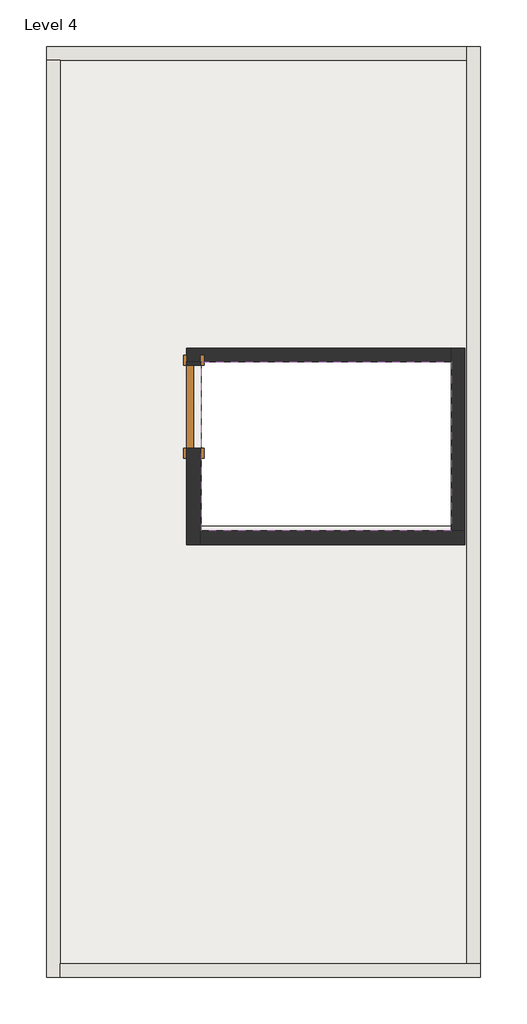
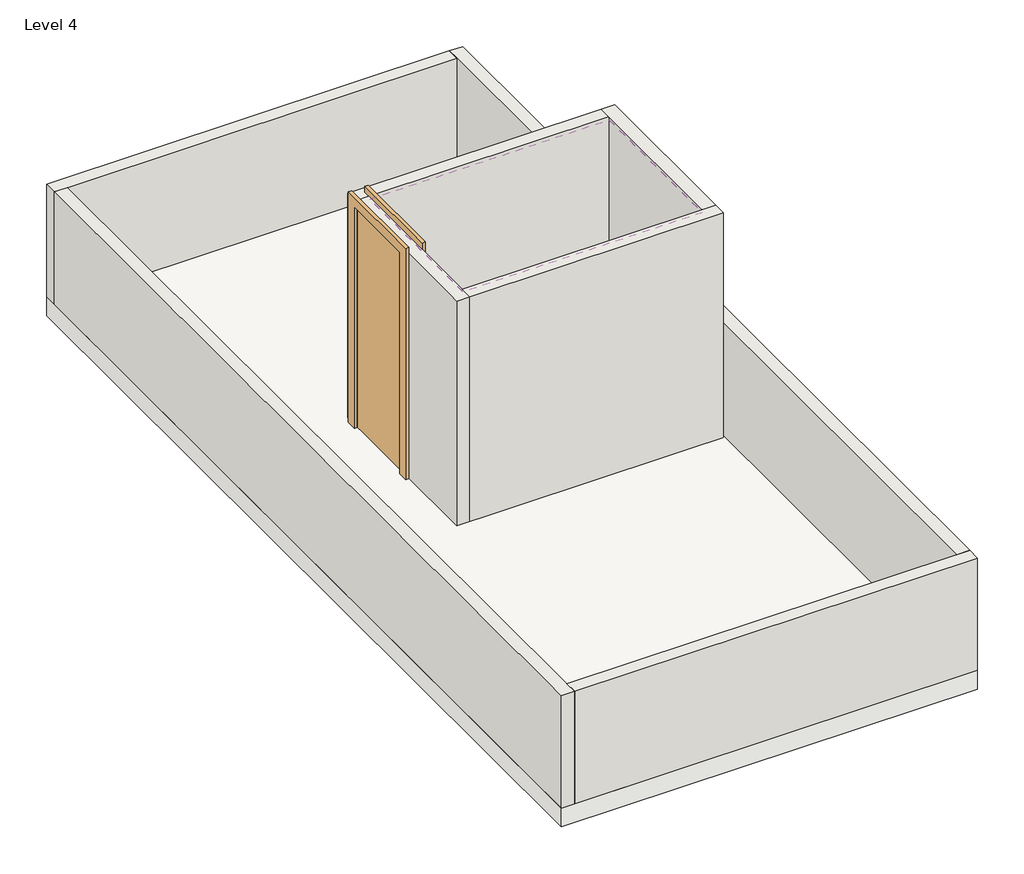
# One storey: 8 walls, 1 covering, 1 door, 1 slab.
"""IFC4 building model written with IfcOpenShell, lengths in millimetres."""

from ifc_helpers import new_model, si_unit, frame, origin, place, context, project, spatial, polyline, outline, extrude, faceted_brep, transform, mapped, element, save
from components import single_flush_2_f3cad073

model = new_model("IFC4")

# Units and contexts
model_context = context("Model", 3, world=origin())
ifc_project = project(units=[si_unit("LENGTHUNIT", "METRE", prefix="MILLI")], contexts=[model_context])

# Site, building, storey
site = spatial("IfcSite", under=ifc_project)
building = spatial("IfcBuilding", under=site)
storey = spatial("IfcBuildingStorey", under=building, Name="Level 4", Elevation=9601.2)

# Covering
placement = place(None, origin())
element("IfcCovering", 1, ObjectType="2' x 4' ACT System", at=placement, inside=storey, context=model_context, shape_type="SweptSolid", body=[
    extrude(outline(polyline([(-2743.5134065, 4950.7083475), (-2743.5134065, 3705.930501), (-4584.856559, 3705.930501), (-4584.856559, 4950.7083475), (-2743.5134065, 4950.7083475)])), frame((0.0, 0.0, 11404.6), z_axis=(0.0, 0.0, 1.0), x_axis=(1.0, 0.0, 0.0)), (0.0, 0.0, 1.0), 57.15),
])

# Door
single_flush_2_shape = single_flush_2_f3cad073(model_context)
element("IfcDoor", 2, ObjectType="Single-Flush : 2'", at=placement, inside=storey, context=model_context, shape_type="MappedRepresentation", body=[
    mapped(single_flush_2_shape, transform((-4642.1634065, 4620.330501, 9601.2), x_axis=(0.0, 1.0, 0.0), y_axis=(-1.0, 0.0, 0.0), z_axis=(0.0, 0.0, 1.0))),
])

# Slab
element("IfcSlab", 3, ObjectType="6\"", at=placement, inside=storey, context=model_context, shape_type="SweptSolid", body=[
    extrude(outline(polyline([(-2527.456559, 7273.2966937), (-2527.456559, 415.2966937), (-5727.856559, 415.2966937), (-5727.856559, 7273.2966937), (-2527.456559, 7273.2966937)]), holes=[polyline([(-4584.856559, 4950.7083475), (-4584.856559, 3743.9980625), (-2711.8237097, 3743.9980625), (-2711.8237097, 4950.7083475), (-4584.856559, 4950.7083475)])]), frame((0.0, 0.0, 9448.8), z_axis=(0.0, 0.0, 1.0), x_axis=(1.0, 0.0, 0.0)), (0.0, 0.0, 1.0), 152.4),
])

# Walls
element("IfcWall", 4, ObjectType="4\"", at=placement, inside=storey, context=model_context, shape_type="Brep", body=[
    faceted_brep([(-5727.856559, 7172.9980625, 9601.2), (-5626.256559, 7172.9980625, 9601.2), (-2629.056559, 7172.9980625, 9601.2), (-2629.056559, 7172.9980625, 10515.6), (-5626.256559, 7172.9980625, 10515.6), (-5727.856559, 7172.9980625, 10515.6), (-5727.856559, 7274.5980625, 9601.2), (-5727.856559, 7274.5980625, 10515.6), (-2629.056559, 7274.5980625, 10515.6), (-2629.056559, 7274.5980625, 9601.2)], [[[0, 1, 2, 3, 4, 5]], [[6, 7, 8, 9]], [[2, 1, 0, 6, 9]], [[5, 4, 3, 8, 7]], [[0, 5, 7, 6]], [[3, 2, 9, 8]]]),
])
element("IfcWall", 5, ObjectType="4\"", at=placement, inside=storey, context=model_context, shape_type="Brep", body=[
    faceted_brep([(-5626.256559, 415.2966937, 9601.2), (-5626.256559, 516.8966937, 9601.2), (-5626.256559, 7172.9980625, 9601.2), (-5626.256559, 7172.9980625, 10515.6), (-5626.256559, 516.8966937, 10515.6), (-5626.256559, 415.2966937, 10515.6), (-5727.856559, 415.2966937, 9601.2), (-5727.856559, 415.2966937, 10515.6), (-5727.856559, 7172.9980625, 10515.6), (-5727.856559, 7172.9980625, 9601.2)], [[[0, 1, 2, 3, 4, 5]], [[6, 7, 8, 9]], [[2, 1, 0, 6, 9]], [[5, 4, 3, 8, 7]], [[0, 5, 7, 6]], [[3, 2, 9, 8]]]),
])
element("IfcWall", 6, ObjectType="4\"", at=placement, inside=storey, context=model_context, shape_type="Brep", body=[
    faceted_brep([(-2527.456559, 516.8966937, 9601.2), (-2629.056559, 516.8966937, 9601.2), (-5626.256559, 516.8966937, 9601.2), (-5626.256559, 516.8966937, 10515.6), (-2629.056559, 516.8966937, 10515.6), (-2527.456559, 516.8966937, 10515.6), (-2527.456559, 415.2966937, 9601.2), (-2527.456559, 415.2966937, 10515.6), (-5626.256559, 415.2966937, 10515.6), (-5626.256559, 415.2966937, 9601.2)], [[[0, 1, 2, 3, 4, 5]], [[6, 7, 8, 9]], [[2, 1, 0, 6, 9]], [[5, 4, 3, 8, 7]], [[0, 5, 7, 6]], [[3, 2, 9, 8]]]),
])
element("IfcWall", 7, ObjectType="4\"", at=placement, inside=storey, context=model_context, shape_type="Brep", body=[
    faceted_brep([(-2629.056559, 7274.5980625, 9601.2), (-2629.056559, 7172.9980625, 9601.2), (-2629.056559, 516.8966937, 9601.2), (-2629.056559, 516.8966937, 10515.6), (-2629.056559, 7172.9980625, 10515.6), (-2629.056559, 7274.5980625, 10515.6), (-2527.456559, 7274.5980625, 9601.2), (-2527.456559, 7274.5980625, 10515.6), (-2527.456559, 516.8966937, 10515.6), (-2527.456559, 516.8966937, 9601.2)], [[[0, 1, 2, 3, 4, 5]], [[6, 7, 8, 9]], [[2, 1, 0, 6, 9]], [[5, 4, 3, 8, 7]], [[0, 5, 7, 6]], [[3, 2, 9, 8]]]),
])
element("IfcWall", 8, ObjectType="4\"", at=placement, inside=storey, context=model_context, shape_type="Brep", body=[
    faceted_brep([(-4692.9634065, 4950.530501, 9601.2), (-4591.3634065, 4950.530501, 9601.2), (-2743.5134065, 4950.530501, 9601.2), (-2743.5134065, 4950.530501, 11430.0), (-4591.3634065, 4950.530501, 11430.0), (-4692.9634065, 4950.530501, 11430.0), (-4692.9634065, 5052.130501, 9601.2), (-4692.9634065, 5052.130501, 11430.0), (-2743.5134065, 5052.130501, 11430.0), (-2743.5134065, 5052.130501, 9601.2)], [[[0, 1, 2, 3, 4, 5]], [[6, 7, 8, 9]], [[2, 1, 0, 6, 9]], [[5, 4, 3, 8, 7]], [[0, 5, 7, 6]], [[3, 2, 9, 8]]]),
])
element("IfcWall", 9, ObjectType="4\"", at=placement, inside=storey, context=model_context, shape_type="Brep", body=[
    faceted_brep([(-4591.3634065, 4950.530501, 11430.0), (-4591.3634065, 3705.930501, 11430.0), (-4591.3634065, 3604.330501, 11430.0), (-4591.3634065, 3604.330501, 9601.2), (-4591.3634065, 3705.930501, 9601.2), (-4591.3634065, 4315.530501, 9601.2), (-4591.3634065, 4315.530501, 11404.6), (-4591.3634065, 4925.130501, 11404.6), (-4591.3634065, 4925.130501, 9601.2), (-4591.3634065, 4950.530501, 9601.2), (-4692.9634065, 3604.330501, 11430.0), (-4692.9634065, 4950.530501, 11430.0), (-4692.9634065, 4950.530501, 9601.2), (-4692.9634065, 4925.130501, 9601.2), (-4692.9634065, 4925.130501, 11404.6), (-4692.9634065, 4315.530501, 11404.6), (-4692.9634065, 4315.530501, 9601.2), (-4692.9634065, 3604.330501, 9601.2)], [[[0, 1, 2, 3, 4, 5, 6, 7, 8, 9]], [[10, 11, 12, 13, 14, 15, 16, 17]], [[3, 17, 16, 5, 4]], [[12, 9, 8, 13]], [[2, 1, 0, 11, 10]], [[3, 2, 10, 17]], [[0, 9, 12, 11]], [[7, 14, 13, 8]], [[14, 7, 6, 15]], [[15, 6, 5, 16]]]),
])
element("IfcWall", 10, ObjectType="4\"", at=placement, inside=storey, context=model_context, shape_type="Brep", body=[
    faceted_brep([(-2641.9134065, 3705.930501, 9601.2), (-2743.5134065, 3705.930501, 9601.2), (-4591.3634065, 3705.930501, 9601.2), (-4591.3634065, 3705.930501, 11430.0), (-2743.5134065, 3705.930501, 11430.0), (-2641.9134065, 3705.930501, 11430.0), (-2641.9134065, 3604.330501, 9601.2), (-2641.9134065, 3604.330501, 11430.0), (-4591.3634065, 3604.330501, 11430.0), (-4591.3634065, 3604.330501, 9601.2)], [[[0, 1, 2, 3, 4, 5]], [[6, 7, 8, 9]], [[2, 1, 0, 6, 9]], [[5, 4, 3, 8, 7]], [[0, 5, 7, 6]], [[3, 2, 9, 8]]]),
])
element("IfcWall", 11, ObjectType="4\"", at=placement, inside=storey, context=model_context, shape_type="Brep", body=[
    faceted_brep([(-2743.5134065, 5052.130501, 9601.2), (-2743.5134065, 4950.530501, 9601.2), (-2743.5134065, 3705.930501, 9601.2), (-2743.5134065, 3705.930501, 11430.0), (-2743.5134065, 4950.530501, 11430.0), (-2743.5134065, 5052.130501, 11430.0), (-2641.9134065, 5052.130501, 9601.2), (-2641.9134065, 5052.130501, 11430.0), (-2641.9134065, 3705.930501, 11430.0), (-2641.9134065, 3705.930501, 9601.2)], [[[0, 1, 2, 3, 4, 5]], [[6, 7, 8, 9]], [[2, 1, 0, 6, 9]], [[5, 4, 3, 8, 7]], [[0, 5, 7, 6]], [[3, 2, 9, 8]]]),
])

save(model, "model.ifc")

# Revit data of these elements
# Type "2' x 4' ACT System"
#   Assembly Code = "C3030210"
#   built-in parameter 1002203 = 1 (stored number, unit not read)
#   built-in parameter 1002202 = 1 (stored number, unit not read)
#   Layers, outside or top first: 0' - 1 5/8" "Default" (function 1); 0' - 0 5/8" "Acoustic Ceiling Tile 24 x 48" (function 5)
# Type "Single-Flush : 2'"
#   Type Mark = "12"
#   Construction Type Id = "MDOOR"
#   Assembly Code = "C1020"
#   Analytic Construction = "Metal"
#   Thickness = 0' - 2"
#   Heat Transfer Coefficient (U) = 0.651978 BTU/(h·ft²·°F)
#   Height = 5' - 11"
#   Trim Projection Ext = 0' - 1"
#   Trim Projection Int = 0' - 1"
#   Trim Width = 0' - 3"
#   Width = 2' - 0"
#   Define Thermal Properties by = 1
#   Door Material = Door - Panel
#   Frame Material = Door - Frame
#   Visual Light Transmittance = 0
#   Solar Heat Gain Coefficient = 0
#   Function = (empty or 0)
#   Wall Closure = (empty or 0)
# Type "6\""
#   Assembly Code = "B1010"
#   Function = 0
#   Layers, outside or top first: 0' - 6" no material (function 1)
# Type "4\""
#   Assembly Code = "B2010"
#   Layers, outside or top first: 0' - 4" no material (function 1)
# Element 1 (IfcCovering, "2' x 4' ACT System")
#   Height Offset From Level = 5' - 11"
#   Phase Created = New Construction
#   Materials on its faces: "Acoustic Ceiling Tile 24 x 48", "Default"
# Element 2 (IfcDoor, "Single-Flush : 2'")
#   Phase Created = New Construction
#   Materials on its faces: "Door - Frame", "Door - Panel"
# Element 3 (IfcSlab, "6\"")
#   Height Offset From Level = 0' - 0"
#   Phase Created = New Construction
#   Materials on its faces: "Default Floor"
# Elements 4, 5, 6, 7 (IfcWall, "4\"")
#   Top Offset = 0' - 0"
#   Base Offset = 0' - 0"
#   Unconnected Height = 3' - 0"
#   wall height = 3' - 0"
#   Phase Created = New Construction
#   Base Constraint = Level 4
#   Materials on its faces: "Default Wall"
# Elements 8, 9, 10, 11 (IfcWall, "4\"")
#   Top Offset = 0' - 0"
#   Base Offset = 0' - 0"
#   Unconnected Height = 6' - 0"
#   wall height = 6' - 0"
#   Phase Created = New Construction
#   Base Constraint = Level 4
#   Materials on its faces: "Default Wall"
# Materials
#   "Default": colour RGB 127 127 127, transparency 0
#   "Acoustic Ceiling Tile 24 x 48": class "Generic", colour RGB 229 229 229, transparency 0, Description = "Acoustic Ceiling Tile 24 x 48", Cost = 0
#   "Door - Panel": class "Wood", colour RGB 210 159 95, transparency 0
#   "Door - Frame": colour RGB 118 70 51, transparency 0
#   "Default Floor": colour RGB 128 128 128, transparency 0
#   "Default Wall": colour RGB 128 128 128, transparency 0
